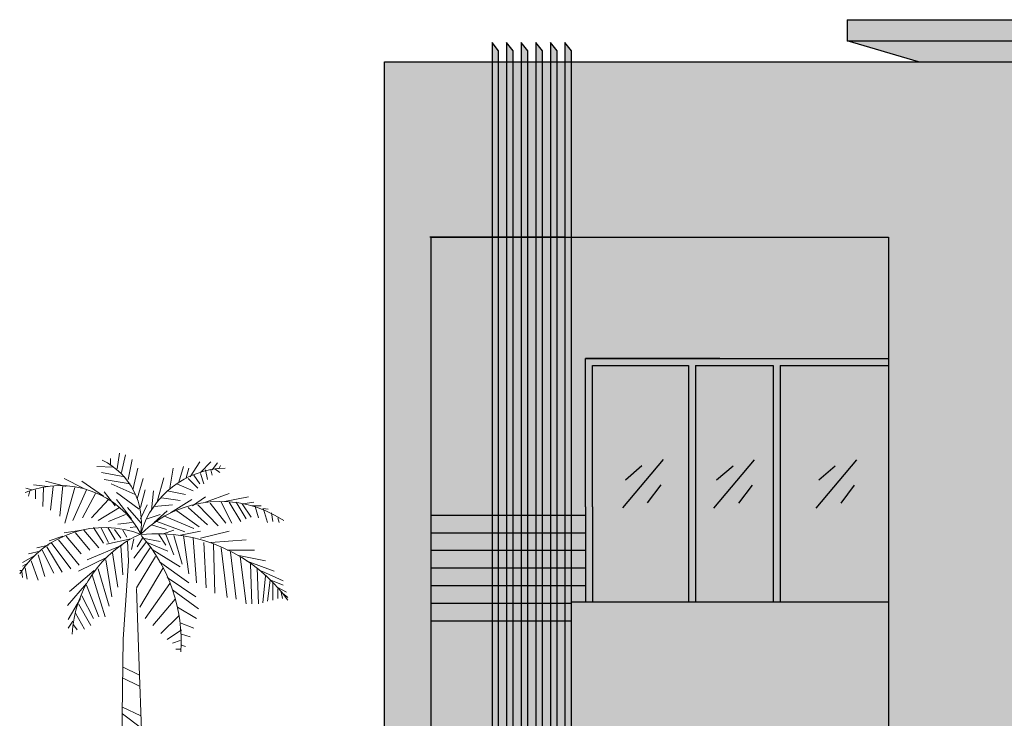
# Model space of a CAD drawing. Units: inches. Extents: x 13 to 1693, y -7 to 1519.
# Tile 6 of 10: x 13 to 292, y 1321 to 1519. Entities that reach past the tile are written whole.
import ezdxf

# ---------------------------------------------------------------- set-up
doc = ezdxf.new("R2010")
doc.units = ezdxf.units.IN
doc.header["$MEASUREMENT"] = 0
for name, color, linetype, lineweight in [('A-ELEV', 7, 'Continuous', 25), ('A-ELEV-PATT', 8, 'Continuous', 13), ('TREE', 102, 'Continuous', 18)]:
    doc.layers.add(name, color=color, linetype=linetype, lineweight=lineweight)

# ---------------------------------------------------------------- blocks, each defined once
blk = doc.blocks.new('*U29')
for p, q in [((-5.567, 196.707), (-4.987, 201.167)), ((-7.5, 199.68), (-7.5, 197.946)), ((-4.407, 195.716), (-3.247, 200.672)), ((-2.474, 193.733), (-1.315, 199.433)), ((15.116, 194.477), (17.822, 198.689)), ((18.015, 195.716), (20.914, 198.689)), ((21.301, 196.459), (22.847, 198.441)), ((-6.727, 197.202), (-11.366, 197.45)), ((-3.441, 194.477), (-10.013, 195.716)), ((-1.121, 190.759), (0.232, 196.955)), ((9.317, 191.255), (10.283, 196.955)), ((11.829, 192.99), (13.182, 197.45)), ((13.956, 194.229), (14.729, 196.955)), ((18.015, 195.468), (18.981, 192.494)), ((19.368, 196.459), (19.948, 193.733)), ((20.914, 196.459), (21.301, 194.972)), ((22.074, 196.707), (23.427, 195.716)), ((23.234, 196.707), (23.62, 197.698)), ((-20.064, 191.751), (-25.863, 193.238)), ((-15.232, 191.255), (-20.644, 193.981)), ((-9.433, 189.025), (-15.618, 193.238)), ((-1.894, 192.494), (-9.24, 193.733)), ((-0.541, 189.52), (-7.307, 192.494)), ((0.038, 188.281), (1.778, 193.981)), ((5.837, 187.786), (7.577, 194.229)), ((11.25, 192.494), (15.889, 190.512)), ((14.536, 193.981), (17.242, 191.255)), ((16.082, 194.972), (17.822, 192.494)), ((-29.729, 190.759), (-31.469, 191.255)), ((-30.309, 190.512), (-30.695, 189.025)), ((-25.283, 191.751), (-29.342, 192.246)), ((-28.763, 190.759), (-28.763, 188.281)), ((-26.443, 191.503), (-26.636, 186.051)), ((-23.737, 191.751), (-24.51, 185.06)), ((-21.031, 191.998), (-21.804, 183.325)), ((-17.551, 191.503), (-20.451, 181.343)), ((-14.265, 190.759), (-18.131, 182.086)), ((-11.753, 189.768), (-15.425, 182.83)), ((-6.147, 186.299), (-9.24, 190.264)), ((-5.76, 190.016), (0.618, 185.308)), ((1.005, 185.803), (2.358, 190.759)), ((4.098, 185.06), (4.678, 190.512)), ((8.544, 190.512), (13.763, 189.52)), ((19.368, 187.29), (26.133, 189.768)), ((-8.08, 188.034), (-12.912, 182.83)), ((-5.76, 188.034), (-1.508, 182.582)), ((6.997, 188.529), (12.216, 187.786)), ((9.51, 184.317), (15.502, 188.034)), ((15.695, 186.299), (19.368, 188.777)), ((20.721, 187.042), (25.167, 181.343)), ((23.814, 187.29), (26.907, 181.343)), ((24.78, 187.538), (31.546, 188.777)), ((26.133, 187.29), (29.419, 181.838)), ((28.066, 187.29), (30.966, 182.582)), ((29.999, 186.795), (33.092, 187.29)), ((-4.987, 185.803), (-10.979, 182.086)), ((-2.668, 185.803), (1.198, 181.343)), ((1.005, 182.582), (2.938, 186.547)), ((4.871, 186.051), (10.09, 186.547)), ((4.871, 181.591), (8.544, 184.812)), ((11.25, 184.812), (17.628, 180.352)), ((14.536, 185.803), (19.948, 180.847)), ((17.242, 186.547), (23.041, 180.599)), ((29.806, 186.795), (32.319, 183.078)), ((32.512, 186.299), (35.218, 186.299)), ((33.479, 186.051), (34.445, 182.83)), ((35.605, 185.556), (37.151, 185.308)), ((35.798, 185.308), (36.958, 181.591)), ((38.118, 184.317), (38.504, 181.838)), ((-3.247, 183.821), (-8.08, 181.838)), ((-1.315, 181.591), (-5.374, 181.095)), ((2.938, 182.582), (6.61, 183.821)), ((5.644, 181.838), (13.569, 178.865)), ((7.77, 183.325), (16.082, 179.856)), ((39.857, 182.83), (40.244, 181.591)), ((-15.618, 179.36), (-20.644, 178.617)), ((-17.358, 178.617), (-13.299, 173.661)), ((-15.038, 179.36), (-10.786, 174.404)), ((-12.332, 180.104), (-9.433, 175.643)), ((-10.206, 180.104), (-8.08, 175.891)), ((-8.273, 180.104), (-6.147, 176.635)), ((-6.34, 179.608), (-4.6, 177.13)), ((-4.021, 179.36), (-2.861, 177.378)), ((-0.348, 180.352), (-1.894, 180.104)), ((4.098, 180.847), (8.35, 179.608)), ((7.384, 178.369), (10.476, 179.36)), ((11.829, 177.874), (18.015, 179.113)), ((18.015, 177.13), (26.133, 179.113)), ((-21.031, 177.626), (-24.897, 176.387)), ((-24.317, 175.891), (-18.711, 168.457)), ((-22.191, 176.635), (-16.391, 169.448)), ((-20.064, 177.626), (-15.812, 172.67)), ((-1.701, 176.882), (-8.66, 175.396)), ((-2.668, 176.387), (-2.376, 170.594)), ((-0.928, 176.882), (-1.508, 173.909)), ((2.551, 175.891), (-0.928, 171.431)), ((1.585, 177.13), (0.038, 174.652)), ((1.585, 177.13), (6.61, 176.139)), ((2.938, 175.891), (8.737, 173.413)), ((6.224, 178.121), (8.157, 175.148)), ((8.157, 178.121), (10.476, 172.422)), ((10.476, 177.874), (12.796, 169.696)), ((13.182, 177.874), (14.729, 166.97)), ((15.889, 177.13), (16.855, 164.492)), ((18.981, 175.891), (19.561, 163.005)), ((20.914, 175.891), (30.966, 176.635)), ((-27.409, 173.413), (-30.695, 172.67)), ((-25.09, 175.148), (-28.376, 174.404)), ((-26.829, 173.661), (-23.544, 167.218)), ((-25.476, 174.652), (-21.224, 167.466)), ((-4.214, 175.148), (-14.072, 170.935)), ((-6.92, 172.917), (-5.374, 163.253)), ((-4.6, 174.9), (-4.021, 166.722)), ((3.711, 174.404), (-0.541, 167.961)), ((4.291, 173.909), (12.216, 168.953)), ((21.688, 175.396), (22.074, 161.518)), ((23.814, 174.404), (25.554, 160.279)), ((25.554, 173.661), (33.285, 173.661)), ((26.52, 173.165), (28.066, 159.784)), ((-28.956, 172.174), (-32.435, 170.192)), ((-29.922, 170.687), (-27.989, 165.235)), ((-27.989, 172.422), (-26.056, 166.227)), ((-8.466, 171.678), (-16.585, 167.713)), ((-8.853, 170.935), (-7.113, 160.527)), ((5.257, 171.926), (-0.155, 163.005)), ((6.417, 170.439), (14.729, 164.492)), ((28.839, 172.174), (36.378, 170.687)), ((29.226, 171.926), (30.966, 158.545)), ((30.966, 170.687), (38.891, 167.713)), ((-32.628, 167.961), (-33.208, 167.961)), ((-32.628, 167.713), (-32.435, 165.979)), ((-31.082, 169.944), (-32.435, 169.2)), ((-31.662, 168.705), (-31.082, 165.483)), ((-12.139, 167.961), (-19.098, 162.014)), ((-10.979, 168.457), (-7.887, 157.801)), ((7.384, 168.705), (0.812, 157.553)), ((32.126, 169.696), (32.512, 158.545)), ((34.058, 168.705), (34.445, 158.545)), ((35.412, 167.713), (41.404, 164.988)), ((-12.719, 166.722), (-9.046, 154.828)), ((8.544, 165.979), (16.662, 160.527)), ((36.378, 166.474), (35.605, 158.792)), ((37.731, 165.235), (36.958, 159.288)), ((37.924, 165.235), (41.404, 163.749)), ((-14.265, 164.244), (-19.678, 158.049)), ((-14.265, 163.749), (-10.786, 154.828)), ((9.317, 164.244), (2.358, 154.332)), ((10.09, 162.51), (17.435, 157.058)), ((38.504, 164.492), (38.504, 159.536)), ((39.664, 163.253), (42.37, 161.766)), ((39.857, 162.757), (39.857, 160.031)), ((40.824, 161.766), (41.21, 160.031)), ((-16.005, 160.031), (-19.484, 154.084)), ((-15.618, 160.775), (-12.332, 154.332)), ((10.863, 159.784), (4.484, 152.35)), ((41.21, 161.518), (42.757, 160.279)), ((-16.585, 158.545), (-13.106, 152.35)), ((11.443, 157.553), (16.855, 154.332)), ((-18.131, 153.589), (-19.484, 151.606)), ((-17.358, 155.819), (-14.845, 151.358)), ((11.829, 155.075), (6.804, 150.119)), ((-17.938, 152.597), (-16.972, 151.111)), ((12.603, 151.111), (8.544, 148.385)), ((12.216, 153.093), (16.082, 151.606)), ((12.216, 148.137), (10.09, 147.393)), ((12.603, 149.872), (15.116, 149.128)), ((12.409, 145.659), (11.056, 145.659)), ((12.409, 146.898), (13.763, 146.402)), ((-4.081, 140.645), (0.753, 138.261)), ((-4.081, 137.547), (0.753, 135.163)), ((-4.081, 129.205), (1.124, 126.821)), ((-4.081, 127.298), (1.31, 123.246)), ((-4.081, 121.578), (1.31, 120.863)), ((-4.267, 114.428), (1.682, 108.708)), ((-4.453, 112.283), (1.682, 105.133)), ((-4.639, 102.273), (1.868, 100.604)), ((-4.453, 99.651), (2.24, 98.459)), ((-4.453, 91.071), (2.426, 89.641)), ((-4.825, 83.921), (2.612, 81.061)), ((-4.639, 81.299), (2.797, 78.916)), ((-4.639, 78.916), (2.797, 76.771))]:
    blk.add_line(p, q)
for points in [[(-2.363, 170.553), (-3.88, 148.505), (-4.988, 69.634), (-3.325, 24.869), (0, 0)], [(-0.116, 162.848), (0.554, 143.532), (2.217, 96.635), (3.88, 44.054), (7.76, 12.079), (11.64, 0)]]:
    blk.add_lwpolyline(points)
for centre, radius, start, end in [((-18.427, 181.448), 19.715, 350.285, 64.11229), ((25.595, 171.567), 25.395, 91.40319, 163.882), ((-21.738, 166.094), 25.899, 27.67115, 112.5305), ((23.687, 155.341), 32.188, 56.19272, 134.3213), ((-9.259, 151.732), 28.386, 68.38311, 147.5322), ((14.394, 148.393), 32.752, 113.7592, 177.4133), ((5.828, 132.718), 45.639, 35.98777, 95.82273), ((-32.8, 147.923), 45.309, 356.1943, 41.37848)]:
    blk.add_arc(centre, radius, start, end)

msp = doc.modelspace()

# ---------------------------------------------------------------- hatches: boundary and pattern name
at = {"layer": 'A-ELEV-PATT'}
h = msp.add_hatch(color=256, dxfattribs=at)
h.dxf.hatch_style = 1
h.paths.add_polyline_path([(526.9, 1519.22), (247.4, 1519.22), (247.4, 1513.22), (526.9, 1513.22)])
at = {"layer": 'A-ELEV-PATT', "transparency": 33554664}
h = msp.add_hatch(color=256, dxfattribs=at)
h.dxf.hatch_style = 1
h.paths.add_polyline_path([(161.14, 1507.23), (159.26, 1507.23), (159.26, 1457.61), (161.14, 1457.61)])
h.paths.add_polyline_path([(161.14, 1510.4), (159.26, 1512.79), (159.26, 1507.23), (161.14, 1507.23)])
h.paths.add_polyline_path([(165.27, 1510.4), (163.39, 1512.79), (163.39, 1507.23), (165.27, 1507.23)])
h.paths.add_polyline_path([(169.4, 1510.4), (167.53, 1512.79), (167.53, 1507.23), (169.4, 1507.23)])
h.paths.add_polyline_path([(157.01, 1510.4), (155.13, 1512.79), (155.13, 1507.23), (157.01, 1507.23)])
h.paths.add_polyline_path([(152.87, 1510.4), (151, 1512.79), (151, 1507.23), (152.87, 1507.23)])
h.paths.add_polyline_path([(148.74, 1510.4), (146.87, 1512.79), (146.87, 1507.23), (148.74, 1507.23)])
h.paths.add_polyline_path([(148.74, 1507.23), (146.87, 1507.23), (146.87, 1457.61), (148.74, 1457.61)])
h.paths.add_polyline_path([(152.87, 1507.23), (151, 1507.23), (151, 1457.61), (152.87, 1457.61)])
h.paths.add_polyline_path([(157.01, 1507.23), (155.13, 1507.23), (155.13, 1457.61), (157.01, 1457.61)])
h.paths.add_polyline_path([(165.27, 1507.23), (163.39, 1507.23), (163.39, 1457.61), (165.27, 1457.61)])
h.paths.add_polyline_path([(169.4, 1507.23), (167.53, 1507.23), (167.53, 1457.61), (169.4, 1457.61)])
h.paths.add_polyline_path([(157.01, 1457.61), (155.13, 1457.61), (155.13, 1213.23), (157.01, 1213.23)])
h.paths.add_polyline_path([(161.14, 1457.61), (159.26, 1457.61), (159.26, 1213.23), (161.14, 1213.23)])
h.paths.add_polyline_path([(165.27, 1457.61), (163.39, 1457.61), (163.39, 1213.23), (165.27, 1213.23)])
h.paths.add_polyline_path([(169.4, 1457.61), (167.53, 1457.61), (167.53, 1213.23), (169.4, 1213.23)])
h.paths.add_polyline_path([(152.87, 1457.61), (151, 1457.61), (151, 1213.23), (152.87, 1213.23)])
h.paths.add_polyline_path([(148.74, 1457.61), (146.87, 1457.61), (146.87, 1213.23), (148.74, 1213.23)])
at = {"layer": 'A-ELEV-PATT'}
h = msp.add_hatch(color=256, dxfattribs=at)
h.dxf.hatch_style = 1
h.paths.add_polyline_path([(485.45, 1459.23), (314.45, 1459.23), (323.77, 1437.38), (485.45, 1437.38)])
h.paths.add_polyline_path([(323.77, 1437.38), (314.45, 1459.23), (314.45, 1204.63), (323.77, 1213.23), (323.77, 1423.23)])
h.paths.add_polyline_path([(526.9, 1513.22), (247.4, 1513.22), (267.64, 1507.23), (519.7, 1507.23)])
h = msp.add_hatch(color=256, dxfattribs=at)
h.dxf.hatch_style = 1
h.paths.add_polyline_path([(534.67, 1493.81), (311.73, 1493.81), (311.73, 1507.23), (169.4, 1507.23), (169.4, 1457.61), (259.19, 1457.61), (259.19, 1213.23), (294.63, 1213.23), (294.63, 1485.7), (299.21, 1485.7), (534.67, 1485.7)])
h.paths.add_polyline_path([(534.67, 1481.12), (299.21, 1481.12), (299.21, 1213.23), (314.45, 1213.23), (314.45, 1459.23), (520.13, 1459.23)], flags=17)
h.paths.add_polyline_path([(146.87, 1507.23), (116.45, 1507.23), (116.45, 1339.23), (116.45, 1213.23), (129.66, 1213.23), (129.66, 1457.61), (146.87, 1457.61)])
h.paths.add_polyline_path([(151, 1507.23), (148.74, 1507.23), (148.74, 1457.61), (151, 1457.61)])
h.paths.add_polyline_path([(155.13, 1507.23), (152.87, 1507.23), (152.87, 1457.61), (155.13, 1457.61)])
h.paths.add_polyline_path([(159.26, 1507.23), (157.01, 1507.23), (157.01, 1457.61), (159.26, 1457.61)])
h.paths.add_polyline_path([(163.39, 1507.23), (161.14, 1507.23), (161.14, 1457.61), (163.39, 1457.61)])
h.paths.add_polyline_path([(167.53, 1507.23), (165.27, 1507.23), (165.27, 1457.61), (167.53, 1457.61)])
h = msp.add_hatch(color=256, dxfattribs=at)
h.dxf.hatch_style = 1
h.paths.add_polyline_path([(259.19, 1457.61), (169.4, 1457.61), (169.4, 1453.8), (259.19, 1453.8)])
h.paths.add_polyline_path([(259.19, 1448.8), (169.4, 1448.8), (169.4, 1443.8), (259.19, 1443.8)])
h.paths.add_polyline_path([(259.19, 1438.8), (169.4, 1438.8), (169.4, 1433.8), (259.19, 1433.8)])
h.paths.add_polyline_path([(259.19, 1428.8), (169.4, 1428.8), (169.4, 1423.8), (259.19, 1423.8)])
h.paths.add_polyline_path([(146.87, 1457.61), (129.66, 1457.61), (129.66, 1453.8), (146.87, 1453.8)])
h.paths.add_polyline_path([(146.87, 1448.8), (129.66, 1448.8), (129.66, 1443.8), (146.87, 1443.8)])
h.paths.add_polyline_path([(146.87, 1438.8), (129.66, 1438.8), (129.66, 1433.8), (146.87, 1433.8)])
h.paths.add_polyline_path([(146.87, 1428.8), (129.66, 1428.8), (129.66, 1423.8), (146.87, 1423.8)])
h.paths.add_polyline_path([(151, 1457.61), (148.74, 1457.61), (148.74, 1453.8), (151, 1453.8)])
h.paths.add_polyline_path([(155.13, 1457.61), (152.87, 1457.61), (152.87, 1453.8), (155.13, 1453.8)])
h.paths.add_polyline_path([(159.26, 1457.61), (157.01, 1457.61), (157.01, 1453.8), (159.26, 1453.8)])
h.paths.add_polyline_path([(163.39, 1457.61), (161.14, 1457.61), (161.14, 1453.8), (163.39, 1453.8)])
h.paths.add_polyline_path([(167.53, 1457.61), (165.27, 1457.61), (165.27, 1453.8), (167.53, 1453.8)])
h.paths.add_polyline_path([(167.53, 1448.8), (165.27, 1448.8), (165.27, 1443.8), (167.53, 1443.8)])
h.paths.add_polyline_path([(163.39, 1448.8), (161.14, 1448.8), (161.14, 1443.8), (163.39, 1443.8)])
h.paths.add_polyline_path([(159.26, 1448.8), (157.01, 1448.8), (157.01, 1443.8), (159.26, 1443.8)])
h.paths.add_polyline_path([(155.13, 1448.8), (152.87, 1448.8), (152.87, 1443.8), (155.13, 1443.8)])
h.paths.add_polyline_path([(151, 1448.8), (148.74, 1448.8), (148.74, 1443.8), (151, 1443.8)])
h.paths.add_polyline_path([(151, 1438.8), (148.74, 1438.8), (148.74, 1433.8), (151, 1433.8)])
h.paths.add_polyline_path([(155.13, 1438.8), (152.87, 1438.8), (152.87, 1433.8), (155.13, 1433.8)])
h.paths.add_polyline_path([(159.26, 1438.8), (157.01, 1438.8), (157.01, 1433.8), (159.26, 1433.8)])
h.paths.add_polyline_path([(163.39, 1438.8), (161.14, 1438.8), (161.14, 1433.8), (163.39, 1433.8)])
h.paths.add_polyline_path([(167.53, 1438.8), (165.27, 1438.8), (165.27, 1433.8), (167.53, 1433.8)])
h.paths.add_polyline_path([(167.53, 1428.8), (165.27, 1428.8), (165.27, 1423.8), (167.53, 1423.8)])
h.paths.add_polyline_path([(163.39, 1428.8), (161.14, 1428.8), (161.14, 1423.8), (163.39, 1423.8)])
h.paths.add_polyline_path([(159.26, 1428.8), (157.01, 1428.8), (157.01, 1423.8), (159.26, 1423.8)])
h.paths.add_polyline_path([(155.13, 1428.8), (152.87, 1428.8), (152.87, 1423.8), (155.13, 1423.8)])
h.paths.add_polyline_path([(151, 1428.8), (148.74, 1428.8), (148.74, 1423.8), (151, 1423.8)])
h.paths.add_polyline_path([(146.87, 1418.8), (129.66, 1418.8), (129.66, 1413.8), (146.87, 1413.8)])
h.paths.add_polyline_path([(146.87, 1408.8), (129.66, 1408.8), (129.66, 1403.8), (146.87, 1403.8)])
h.paths.add_polyline_path([(146.87, 1398.8), (129.66, 1398.8), (129.66, 1393.8), (146.87, 1393.8)])
h.paths.add_polyline_path([(146.87, 1388.8), (129.66, 1388.8), (129.66, 1383.8), (146.87, 1383.8)])
h.paths.add_polyline_path([(146.87, 1378.8), (129.66, 1378.8), (129.66, 1373.8), (146.87, 1373.8)])
h.paths.add_polyline_path([(146.87, 1368.8), (129.66, 1368.8), (129.66, 1363.8), (146.87, 1363.8)])
h.paths.add_polyline_path([(146.87, 1358.8), (129.66, 1358.8), (129.66, 1353.8), (146.87, 1353.8)])
h.paths.add_polyline_path([(146.87, 1348.8), (129.66, 1348.8), (129.66, 1343.8), (146.87, 1343.8)])
h.paths.add_polyline_path([(146.87, 1338.8), (129.66, 1338.8), (129.66, 1333.8), (146.87, 1333.8)])
h.paths.add_polyline_path([(146.87, 1328.8), (129.66, 1328.8), (129.66, 1323.8), (146.87, 1323.8)])
h.paths.add_polyline_path([(146.87, 1318.8), (129.66, 1318.8), (129.66, 1312.21), (146.87, 1312.21)])
h.paths.add_polyline_path([(146.87, 1307.21), (129.66, 1307.21), (129.66, 1302.21), (146.87, 1302.21)])
h.paths.add_polyline_path([(146.87, 1297.21), (129.66, 1297.21), (129.66, 1292.21), (146.87, 1292.21)])
h.paths.add_polyline_path([(146.87, 1287.21), (129.66, 1287.21), (129.66, 1282.21), (146.87, 1282.21)])
h.paths.add_polyline_path([(146.87, 1277.21), (129.66, 1277.21), (129.66, 1272.21), (146.87, 1272.21)])
h.paths.add_polyline_path([(146.87, 1267.21), (129.66, 1267.21), (129.66, 1262.21), (146.87, 1262.21)])
h.paths.add_polyline_path([(146.87, 1257.21), (129.66, 1257.21), (129.66, 1252.21), (146.87, 1252.21)])
h.paths.add_polyline_path([(146.87, 1247.21), (129.66, 1247.21), (129.66, 1242.21), (146.87, 1242.21)])
h = msp.add_hatch(color=256, dxfattribs=at)
h.dxf.hatch_style = 1
h.paths.add_polyline_path([(259.19, 1453.8), (169.4, 1453.8), (169.4, 1448.8), (259.19, 1448.8)])
h.paths.add_polyline_path([(259.19, 1443.8), (169.4, 1443.8), (169.4, 1438.8), (259.19, 1438.8)])
h.paths.add_polyline_path([(259.19, 1433.8), (169.4, 1433.8), (169.4, 1428.8), (259.19, 1428.8)])
h.paths.add_polyline_path([(146.87, 1453.8), (129.66, 1453.8), (129.66, 1448.8), (146.87, 1448.8)])
h.paths.add_polyline_path([(146.87, 1443.8), (129.66, 1443.8), (129.66, 1438.8), (146.87, 1438.8)])
h.paths.add_polyline_path([(146.87, 1433.8), (129.66, 1433.8), (129.66, 1428.8), (146.87, 1428.8)])
h.paths.add_polyline_path([(146.87, 1423.8), (129.66, 1423.8), (129.66, 1418.8), (146.87, 1418.8)])
h.paths.add_polyline_path([(146.87, 1413.8), (129.66, 1413.8), (129.66, 1408.8), (146.87, 1408.8)])
h.paths.add_polyline_path([(146.87, 1403.8), (129.66, 1403.8), (129.66, 1398.8), (146.87, 1398.8)])
h.paths.add_polyline_path([(146.87, 1393.8), (129.66, 1393.8), (129.66, 1388.8), (146.87, 1388.8)])
h.paths.add_polyline_path([(146.87, 1383.8), (129.66, 1383.8), (129.66, 1378.8), (146.87, 1378.8)])
h.paths.add_polyline_path([(146.87, 1373.8), (129.66, 1373.8), (129.66, 1368.8), (146.87, 1368.8)])
h.paths.add_polyline_path([(146.87, 1363.8), (129.66, 1363.8), (129.66, 1358.8), (146.87, 1358.8)])
h.paths.add_polyline_path([(146.87, 1353.8), (129.66, 1353.8), (129.66, 1348.8), (146.87, 1348.8)])
h.paths.add_polyline_path([(146.87, 1343.8), (129.66, 1343.8), (129.66, 1338.8), (146.87, 1338.8)])
h.paths.add_polyline_path([(146.87, 1333.8), (129.66, 1333.8), (129.66, 1328.8), (146.87, 1328.8)])
h.paths.add_polyline_path([(146.87, 1323.8), (129.66, 1323.8), (129.66, 1318.8), (146.87, 1318.8)])
h.paths.add_polyline_path([(146.87, 1312.21), (129.66, 1312.21), (129.66, 1307.21), (146.87, 1307.21)])
h.paths.add_polyline_path([(146.87, 1302.21), (129.66, 1302.21), (129.66, 1297.21), (146.87, 1297.21)])
h.paths.add_polyline_path([(146.87, 1292.21), (129.66, 1292.21), (129.66, 1287.21), (146.87, 1287.21)])
h.paths.add_polyline_path([(146.87, 1282.21), (129.66, 1282.21), (129.66, 1277.21), (146.87, 1277.21)])
h.paths.add_polyline_path([(146.87, 1272.21), (129.66, 1272.21), (129.66, 1267.21), (146.87, 1267.21)])
h.paths.add_polyline_path([(146.87, 1262.21), (129.66, 1262.21), (129.66, 1257.21), (146.87, 1257.21)])
h.paths.add_polyline_path([(146.87, 1252.21), (129.66, 1252.21), (129.66, 1247.21), (146.87, 1247.21)])
h.paths.add_polyline_path([(146.87, 1242.21), (129.66, 1242.21), (129.66, 1237.21), (146.87, 1237.21)])
h.paths.add_polyline_path([(146.87, 1232.21), (129.66, 1232.21), (129.66, 1227.21), (146.87, 1227.21)])
h.paths.add_polyline_path([(146.87, 1222.21), (129.66, 1222.21), (129.66, 1217.21), (146.87, 1217.21)])
h.paths.add_polyline_path([(259.19, 1242.21), (169.4, 1242.21), (169.4, 1237.21), (259.19, 1237.21)])
h.paths.add_polyline_path([(259.19, 1232.21), (169.4, 1232.21), (169.4, 1227.21), (259.19, 1227.21)])
h.paths.add_polyline_path([(259.19, 1222.21), (169.4, 1222.21), (169.4, 1217.21), (259.19, 1217.21)])
h = msp.add_hatch(color=256, dxfattribs=at)
h.dxf.hatch_style = 1
h.paths.add_polyline_path([(173.34, 1282.21), (169.4, 1282.21), (169.4, 1277.21), (173.34, 1277.21)])
h.paths.add_polyline_path([(173.34, 1292.21), (169.4, 1292.21), (169.4, 1287.21), (173.34, 1287.21)])
h.paths.add_polyline_path([(173.34, 1272.21), (169.4, 1272.21), (169.4, 1267.21), (173.34, 1267.21)])
h.paths.add_polyline_path([(173.34, 1262.21), (169.4, 1262.21), (169.4, 1257.21), (173.34, 1257.21)])
h.paths.add_polyline_path([(173.34, 1312.21), (169.4, 1312.21), (169.4, 1307.21), (173.34, 1307.21)])
h.paths.add_polyline_path([(173.34, 1302.21), (169.4, 1302.21), (169.4, 1297.21), (173.34, 1297.21)])
h.paths.add_polyline_path([(167.53, 1323.8), (165.27, 1323.8), (165.27, 1318.8), (167.53, 1318.8)])
h.paths.add_polyline_path([(167.53, 1333.8), (165.27, 1333.8), (165.27, 1328.8), (167.53, 1328.8)])
h.paths.add_polyline_path([(163.39, 1333.8), (161.14, 1333.8), (161.14, 1328.8), (163.39, 1328.8)])
h.paths.add_polyline_path([(159.26, 1333.8), (157.01, 1333.8), (157.01, 1328.8), (159.26, 1328.8)])
h.paths.add_polyline_path([(155.13, 1333.8), (152.87, 1333.8), (152.87, 1328.8), (155.13, 1328.8)])
h.paths.add_polyline_path([(151, 1333.8), (148.74, 1333.8), (148.74, 1328.8), (151, 1328.8)])
h.paths.add_polyline_path([(151, 1323.8), (148.74, 1323.8), (148.74, 1318.8), (151, 1318.8)])
h.paths.add_polyline_path([(155.13, 1323.8), (152.87, 1323.8), (152.87, 1318.8), (155.13, 1318.8)])
h.paths.add_polyline_path([(159.26, 1323.8), (157.01, 1323.8), (157.01, 1318.8), (159.26, 1318.8)])
h.paths.add_polyline_path([(163.39, 1323.8), (161.14, 1323.8), (161.14, 1318.8), (163.39, 1318.8)])
h.paths.add_polyline_path([(163.39, 1312.21), (161.14, 1312.21), (161.14, 1307.21), (163.39, 1307.21)])
h.paths.add_polyline_path([(167.53, 1312.21), (165.27, 1312.21), (165.27, 1307.21), (167.53, 1307.21)])
h.paths.add_polyline_path([(167.53, 1302.21), (165.27, 1302.21), (165.27, 1297.21), (167.53, 1297.21)])
h.paths.add_polyline_path([(167.53, 1292.21), (165.27, 1292.21), (165.27, 1287.21), (167.53, 1287.21)])
h.paths.add_polyline_path([(163.39, 1292.21), (161.14, 1292.21), (161.14, 1287.21), (163.39, 1287.21)])
h.paths.add_polyline_path([(163.39, 1302.21), (161.14, 1302.21), (161.14, 1297.21), (163.39, 1297.21)])
h.paths.add_polyline_path([(159.26, 1302.21), (157.01, 1302.21), (157.01, 1297.21), (159.26, 1297.21)])
h.paths.add_polyline_path([(159.26, 1312.21), (157.01, 1312.21), (157.01, 1307.21), (159.26, 1307.21)])
h.paths.add_polyline_path([(155.13, 1312.21), (152.87, 1312.21), (152.87, 1307.21), (155.13, 1307.21)])
h.paths.add_polyline_path([(151, 1312.21), (148.74, 1312.21), (148.74, 1307.21), (151, 1307.21)])
h.paths.add_polyline_path([(151, 1302.21), (148.74, 1302.21), (148.74, 1297.21), (151, 1297.21)])
h.paths.add_polyline_path([(155.13, 1302.21), (152.87, 1302.21), (152.87, 1297.21), (155.13, 1297.21)])
h.paths.add_polyline_path([(155.13, 1292.21), (152.87, 1292.21), (152.87, 1287.21), (155.13, 1287.21)])
h.paths.add_polyline_path([(151, 1292.21), (148.74, 1292.21), (148.74, 1287.21), (151, 1287.21)])
h.paths.add_polyline_path([(159.26, 1292.21), (157.01, 1292.21), (157.01, 1287.21), (159.26, 1287.21)])
h.paths.add_polyline_path([(159.26, 1282.21), (157.01, 1282.21), (157.01, 1277.21), (159.26, 1277.21)])
h.paths.add_polyline_path([(163.39, 1282.21), (161.14, 1282.21), (161.14, 1277.21), (163.39, 1277.21)])
h.paths.add_polyline_path([(167.53, 1282.21), (165.27, 1282.21), (165.27, 1277.21), (167.53, 1277.21)])
h.paths.add_polyline_path([(155.13, 1282.21), (152.87, 1282.21), (152.87, 1277.21), (155.13, 1277.21)])
h.paths.add_polyline_path([(151, 1282.21), (148.74, 1282.21), (148.74, 1277.21), (151, 1277.21)])
h.paths.add_polyline_path([(151, 1272.21), (148.74, 1272.21), (148.74, 1267.21), (151, 1267.21)])
h.paths.add_polyline_path([(155.13, 1272.21), (152.87, 1272.21), (152.87, 1267.21), (155.13, 1267.21)])
h.paths.add_polyline_path([(159.26, 1272.21), (157.01, 1272.21), (157.01, 1267.21), (159.26, 1267.21)])
h.paths.add_polyline_path([(163.39, 1272.21), (161.14, 1272.21), (161.14, 1267.21), (163.39, 1267.21)])
h.paths.add_polyline_path([(167.53, 1272.21), (165.27, 1272.21), (165.27, 1267.21), (167.53, 1267.21)])
h.paths.add_polyline_path([(167.53, 1262.21), (165.27, 1262.21), (165.27, 1257.21), (167.53, 1257.21)])
h.paths.add_polyline_path([(163.39, 1262.21), (161.14, 1262.21), (161.14, 1257.21), (163.39, 1257.21)])
h.paths.add_polyline_path([(163.39, 1252.21), (161.14, 1252.21), (161.14, 1247.21), (163.39, 1247.21)])
h.paths.add_polyline_path([(159.26, 1252.21), (157.01, 1252.21), (157.01, 1247.21), (159.26, 1247.21)])
h.paths.add_polyline_path([(159.26, 1262.21), (157.01, 1262.21), (157.01, 1257.21), (159.26, 1257.21)])
h.paths.add_polyline_path([(155.13, 1262.21), (152.87, 1262.21), (152.87, 1257.21), (155.13, 1257.21)])
h.paths.add_polyline_path([(151, 1262.21), (148.74, 1262.21), (148.74, 1257.21), (151, 1257.21)])
h.paths.add_polyline_path([(151, 1252.21), (148.74, 1252.21), (148.74, 1247.21), (151, 1247.21)])
h.paths.add_polyline_path([(155.13, 1252.21), (152.87, 1252.21), (152.87, 1247.21), (155.13, 1247.21)])
h.paths.add_polyline_path([(151, 1242.21), (148.74, 1242.21), (148.74, 1237.21), (151, 1237.21)])
h.paths.add_polyline_path([(155.13, 1242.21), (152.87, 1242.21), (152.87, 1237.21), (155.13, 1237.21)])
h.paths.add_polyline_path([(159.26, 1242.21), (157.01, 1242.21), (157.01, 1237.21), (159.26, 1237.21)])
h.paths.add_polyline_path([(163.39, 1242.21), (161.14, 1242.21), (161.14, 1237.21), (163.39, 1237.21)])
h.paths.add_polyline_path([(173.34, 1363.8), (169.4, 1363.8), (169.4, 1358.8), (173.34, 1358.8)])
h.paths.add_polyline_path([(173.34, 1373.8), (169.4, 1373.8), (169.4, 1368.8), (173.34, 1368.8)])
h.paths.add_polyline_path([(173.34, 1381.23), (173.34, 1383.8), (169.4, 1383.8), (169.4, 1378.8), (173.34, 1378.8)])
h.paths.add_polyline_path([(173.34, 1393.8), (169.4, 1393.8), (169.4, 1388.8), (173.34, 1388.8)])
h.paths.add_polyline_path([(173.34, 1403.8), (169.4, 1403.8), (169.4, 1398.8), (173.34, 1398.8)])
h.paths.add_polyline_path([(173.34, 1413.8), (169.4, 1413.8), (169.4, 1408.8), (173.34, 1408.8)])
h.paths.add_polyline_path([(167.53, 1383.8), (165.27, 1383.8), (165.27, 1378.8), (167.53, 1378.8)])
h.paths.add_polyline_path([(167.53, 1373.8), (165.27, 1373.8), (165.27, 1368.8), (167.53, 1368.8)])
h.paths.add_polyline_path([(167.53, 1363.8), (165.27, 1363.8), (165.27, 1358.8), (167.53, 1358.8)])
h.paths.add_polyline_path([(167.53, 1353.8), (165.27, 1353.8), (165.27, 1348.8), (167.53, 1348.8)])
h.paths.add_polyline_path([(163.39, 1353.8), (161.14, 1353.8), (161.14, 1348.8), (163.39, 1348.8)])
h.paths.add_polyline_path([(163.39, 1363.8), (161.14, 1363.8), (161.14, 1358.8), (163.39, 1358.8)])
h.paths.add_polyline_path([(163.39, 1373.8), (161.14, 1373.8), (161.14, 1368.8), (163.39, 1368.8)])
h.paths.add_polyline_path([(163.39, 1383.8), (161.14, 1383.8), (161.14, 1378.8), (163.39, 1378.8)])
h.paths.add_polyline_path([(163.39, 1393.8), (161.14, 1393.8), (161.14, 1388.8), (163.39, 1388.8)])
h.paths.add_polyline_path([(163.39, 1403.8), (161.14, 1403.8), (161.14, 1398.8), (163.39, 1398.8)])
h.paths.add_polyline_path([(167.53, 1403.8), (165.27, 1403.8), (165.27, 1398.8), (167.53, 1398.8)])
h.paths.add_polyline_path([(167.53, 1393.8), (165.27, 1393.8), (165.27, 1388.8), (167.53, 1388.8)])
h.paths.add_polyline_path([(167.53, 1413.8), (165.27, 1413.8), (165.27, 1408.8), (167.53, 1408.8)])
h.paths.add_polyline_path([(163.39, 1413.8), (161.14, 1413.8), (161.14, 1408.8), (163.39, 1408.8)])
h.paths.add_polyline_path([(159.26, 1413.8), (157.01, 1413.8), (157.01, 1408.8), (159.26, 1408.8)])
h.paths.add_polyline_path([(155.13, 1413.8), (152.87, 1413.8), (152.87, 1408.8), (155.13, 1408.8)])
h.paths.add_polyline_path([(151, 1413.8), (148.74, 1413.8), (148.74, 1408.8), (151, 1408.8)])
h.paths.add_polyline_path([(151, 1403.8), (148.74, 1403.8), (148.74, 1398.8), (151, 1398.8)])
h.paths.add_polyline_path([(155.13, 1403.8), (152.87, 1403.8), (152.87, 1398.8), (155.13, 1398.8)])
h.paths.add_polyline_path([(159.26, 1403.8), (157.01, 1403.8), (157.01, 1398.8), (159.26, 1398.8)])
h.paths.add_polyline_path([(159.26, 1393.8), (157.01, 1393.8), (157.01, 1388.8), (159.26, 1388.8)])
h.paths.add_polyline_path([(155.13, 1393.8), (152.87, 1393.8), (152.87, 1388.8), (155.13, 1388.8)])
h.paths.add_polyline_path([(151, 1393.8), (148.74, 1393.8), (148.74, 1388.8), (151, 1388.8)])
h.paths.add_polyline_path([(151, 1383.8), (148.74, 1383.8), (148.74, 1378.8), (151, 1378.8)])
h.paths.add_polyline_path([(155.13, 1383.8), (152.87, 1383.8), (152.87, 1378.8), (155.13, 1378.8)])
h.paths.add_polyline_path([(159.26, 1383.8), (157.01, 1383.8), (157.01, 1378.8), (159.26, 1378.8)])
h.paths.add_polyline_path([(159.26, 1373.8), (157.01, 1373.8), (157.01, 1368.8), (159.26, 1368.8)])
h.paths.add_polyline_path([(155.13, 1373.8), (152.87, 1373.8), (152.87, 1368.8), (155.13, 1368.8)])
h.paths.add_polyline_path([(151, 1373.8), (148.74, 1373.8), (148.74, 1368.8), (151, 1368.8)])
h.paths.add_polyline_path([(151, 1363.8), (148.74, 1363.8), (148.74, 1358.8), (151, 1358.8)])
h.paths.add_polyline_path([(155.13, 1363.8), (152.87, 1363.8), (152.87, 1358.8), (155.13, 1358.8)])
h.paths.add_polyline_path([(159.26, 1363.8), (157.01, 1363.8), (157.01, 1358.8), (159.26, 1358.8)])
h.paths.add_polyline_path([(159.26, 1353.8), (157.01, 1353.8), (157.01, 1348.8), (159.26, 1348.8)])
h.paths.add_polyline_path([(155.13, 1353.8), (152.87, 1353.8), (152.87, 1348.8), (155.13, 1348.8)])
h.paths.add_polyline_path([(151, 1353.8), (148.74, 1353.8), (148.74, 1348.8), (151, 1348.8)])
h.paths.add_polyline_path([(151, 1343.8), (148.74, 1343.8), (148.74, 1338.8), (151, 1338.8)])
h.paths.add_polyline_path([(155.13, 1343.8), (152.87, 1343.8), (152.87, 1338.8), (155.13, 1338.8)])
h.paths.add_polyline_path([(159.26, 1343.8), (157.01, 1343.8), (157.01, 1338.8), (159.26, 1338.8)])
h.paths.add_polyline_path([(163.39, 1343.8), (161.14, 1343.8), (161.14, 1338.8), (163.39, 1338.8)])
h.paths.add_polyline_path([(167.53, 1343.8), (165.27, 1343.8), (165.27, 1338.8), (167.53, 1338.8)])
h.paths.add_polyline_path([(151, 1453.8), (148.74, 1453.8), (148.74, 1448.8), (151, 1448.8)])
h.paths.add_polyline_path([(155.13, 1453.8), (152.87, 1453.8), (152.87, 1448.8), (155.13, 1448.8)])
h.paths.add_polyline_path([(159.26, 1453.8), (157.01, 1453.8), (157.01, 1448.8), (159.26, 1448.8)])
h.paths.add_polyline_path([(163.39, 1453.8), (161.14, 1453.8), (161.14, 1448.8), (163.39, 1448.8)])
h.paths.add_polyline_path([(167.53, 1453.8), (165.27, 1453.8), (165.27, 1448.8), (167.53, 1448.8)])
h.paths.add_polyline_path([(167.53, 1443.8), (165.27, 1443.8), (165.27, 1438.8), (167.53, 1438.8)])
h.paths.add_polyline_path([(163.39, 1443.8), (161.14, 1443.8), (161.14, 1438.8), (163.39, 1438.8)])
h.paths.add_polyline_path([(159.26, 1443.8), (157.01, 1443.8), (157.01, 1438.8), (159.26, 1438.8)])
h.paths.add_polyline_path([(155.13, 1443.8), (152.87, 1443.8), (152.87, 1438.8), (155.13, 1438.8)])
h.paths.add_polyline_path([(151, 1443.8), (148.74, 1443.8), (148.74, 1438.8), (151, 1438.8)])
h.paths.add_polyline_path([(151, 1433.8), (148.74, 1433.8), (148.74, 1428.8), (151, 1428.8)])
h.paths.add_polyline_path([(155.13, 1433.8), (152.87, 1433.8), (152.87, 1428.8), (155.13, 1428.8)])
h.paths.add_polyline_path([(159.26, 1433.8), (157.01, 1433.8), (157.01, 1428.8), (159.26, 1428.8)])
h.paths.add_polyline_path([(163.39, 1433.8), (161.14, 1433.8), (161.14, 1428.8), (163.39, 1428.8)])
h.paths.add_polyline_path([(167.53, 1433.8), (165.27, 1433.8), (165.27, 1428.8), (167.53, 1428.8)])
h.paths.add_polyline_path([(173.34, 1423.23), (249.37, 1423.23), (259.19, 1423.23), (259.19, 1423.8), (169.4, 1423.8), (169.4, 1418.8), (173.34, 1418.8)])
h.paths.add_polyline_path([(167.53, 1423.8), (165.27, 1423.8), (165.27, 1418.8), (167.53, 1418.8)])
h.paths.add_polyline_path([(163.39, 1423.8), (161.14, 1423.8), (161.14, 1418.8), (163.39, 1418.8)])
h.paths.add_polyline_path([(159.26, 1423.8), (157.01, 1423.8), (157.01, 1418.8), (159.26, 1418.8)])
h.paths.add_polyline_path([(155.13, 1423.8), (152.87, 1423.8), (152.87, 1418.8), (155.13, 1418.8)])
h.paths.add_polyline_path([(151, 1423.8), (148.74, 1423.8), (148.74, 1418.8), (151, 1418.8)])
h = msp.add_hatch(color=256, dxfattribs=at)
h.dxf.hatch_style = 1
h.paths.add_polyline_path([(204.48, 1421.23), (226.48, 1421.23), (226.48, 1354.34), (228.48, 1354.34), (228.48, 1421.23), (259.19, 1421.23), (259.19, 1423.23), (211.36, 1423.23), (173.34, 1423.23), (173.34, 1381.23), (173.34, 1354.34), (175.34, 1354.34), (175.34, 1381.23), (175.34, 1421.23), (202.48, 1421.23), (202.48, 1354.34), (204.48, 1354.34)])
at = {"layer": 'A-ELEV-PATT', "transparency": 33554592}
h = msp.add_hatch(color=256, dxfattribs=at)
h.dxf.hatch_style = 1
h.paths.add_polyline_path([(202.48, 1421.23), (175.34, 1421.23), (175.34, 1381.23), (175.34, 1354.34), (202.48, 1354.34)])
h.paths.add_polyline_path([(226.48, 1421.23), (211.36, 1421.23), (204.48, 1421.23), (204.48, 1354.34), (226.48, 1354.34)])
h.paths.add_polyline_path([(259.19, 1421.23), (228.48, 1421.23), (228.48, 1354.34), (259.19, 1354.34)])
h.paths.add_polyline_path([(259.19, 1316.67), (230.48, 1316.67), (230.48, 1251.23), (259.19, 1251.23)])
h.paths.add_polyline_path([(228.48, 1316.67), (206.48, 1316.67), (206.48, 1251.23), (228.48, 1251.23)])
h.paths.add_polyline_path([(204.48, 1316.67), (175.34, 1316.67), (175.34, 1297.23), (175.34, 1251.23), (204.48, 1251.23)])
h.paths.add_polyline_path([(480.46, 1381.23), (476.14, 1387.14), (476.14, 1345.14), (480.46, 1339.23)])
h.paths.add_polyline_path([(683.45, 1381.23), (480.46, 1381.23), (480.46, 1339.23), (683.45, 1339.23)])
h.paths.add_polyline_path([(348.45, 1421.23), (325.77, 1421.23), (325.77, 1356.34), (348.45, 1356.34)])
h.paths.add_polyline_path([(474.14, 1421.23), (451.45, 1421.23), (451.45, 1356.34), (474.14, 1356.34)])
h.paths.add_polyline_path([(474.14, 1354.34), (451.45, 1354.34), (451.45, 1316.67), (474.14, 1316.67)])
h.paths.add_polyline_path([(348.45, 1354.34), (325.77, 1354.34), (325.77, 1316.67), (348.45, 1316.67)])
h.paths.add_polyline_path([(348.45, 1314.67), (325.77, 1314.67), (325.77, 1215.23), (348.45, 1215.23)])
h.paths.add_polyline_path([(474.14, 1314.67), (451.45, 1314.67), (451.45, 1215.23), (474.14, 1215.23)])
at = {"layer": 'A-ELEV-PATT'}
h = msp.add_hatch(color=256, dxfattribs=at)
h.dxf.hatch_style = 1
h.paths.add_polyline_path([(151, 1418.8), (148.74, 1418.8), (148.74, 1413.8), (151, 1413.8)])
h.paths.add_polyline_path([(155.13, 1418.8), (152.87, 1418.8), (152.87, 1413.8), (155.13, 1413.8)])
h.paths.add_polyline_path([(159.26, 1418.8), (157.01, 1418.8), (157.01, 1413.8), (159.26, 1413.8)])
h.paths.add_polyline_path([(163.39, 1418.8), (161.14, 1418.8), (161.14, 1413.8), (163.39, 1413.8)])
h.paths.add_polyline_path([(167.53, 1418.8), (165.27, 1418.8), (165.27, 1413.8), (167.53, 1413.8)])
h.paths.add_polyline_path([(167.53, 1408.8), (165.27, 1408.8), (165.27, 1403.8), (167.53, 1403.8)])
h.paths.add_polyline_path([(167.53, 1398.8), (165.27, 1398.8), (165.27, 1393.8), (167.53, 1393.8)])
h.paths.add_polyline_path([(167.53, 1388.8), (165.27, 1388.8), (165.27, 1383.8), (167.53, 1383.8)])
h.paths.add_polyline_path([(163.39, 1388.8), (161.14, 1388.8), (161.14, 1383.8), (163.39, 1383.8)])
h.paths.add_polyline_path([(163.39, 1398.8), (161.14, 1398.8), (161.14, 1393.8), (163.39, 1393.8)])
h.paths.add_polyline_path([(163.39, 1408.8), (161.14, 1408.8), (161.14, 1403.8), (163.39, 1403.8)])
h.paths.add_polyline_path([(159.26, 1408.8), (157.01, 1408.8), (157.01, 1403.8), (159.26, 1403.8)])
h.paths.add_polyline_path([(155.13, 1408.8), (152.87, 1408.8), (152.87, 1403.8), (155.13, 1403.8)])
h.paths.add_polyline_path([(151, 1408.8), (148.74, 1408.8), (148.74, 1403.8), (151, 1403.8)])
h.paths.add_polyline_path([(151, 1398.8), (148.74, 1398.8), (148.74, 1393.8), (151, 1393.8)])
h.paths.add_polyline_path([(155.13, 1398.8), (152.87, 1398.8), (152.87, 1393.8), (155.13, 1393.8)])
h.paths.add_polyline_path([(159.26, 1398.8), (157.01, 1398.8), (157.01, 1393.8), (159.26, 1393.8)])
h.paths.add_polyline_path([(159.26, 1388.8), (157.01, 1388.8), (157.01, 1383.8), (159.26, 1383.8)])
h.paths.add_polyline_path([(155.13, 1388.8), (152.87, 1388.8), (152.87, 1383.8), (155.13, 1383.8)])
h.paths.add_polyline_path([(151, 1388.8), (148.74, 1388.8), (148.74, 1383.8), (151, 1383.8)])
h = msp.add_hatch(color=256, dxfattribs=at)
h.dxf.hatch_style = 1
h.paths.add_polyline_path([(173.34, 1398.8), (169.4, 1398.8), (169.4, 1393.8), (173.34, 1393.8)])
h.paths.add_polyline_path([(173.34, 1408.8), (169.4, 1408.8), (169.4, 1403.8), (173.34, 1403.8)])
h.paths.add_polyline_path([(173.34, 1418.8), (169.4, 1418.8), (169.4, 1413.8), (173.34, 1413.8)])
h = msp.add_hatch(color=256, dxfattribs=at)
h.dxf.hatch_style = 1
h.paths.add_polyline_path([(146.87, 1237.21), (129.66, 1237.21), (129.66, 1232.21), (146.87, 1232.21)])
h.paths.add_polyline_path([(146.87, 1227.21), (129.66, 1227.21), (129.66, 1222.21), (146.87, 1222.21)])
h.paths.add_polyline_path([(146.87, 1217.21), (129.66, 1217.21), (129.66, 1213.23), (146.87, 1213.23)])
h.paths.add_polyline_path([(259.19, 1217.21), (169.4, 1217.21), (169.4, 1213.23), (259.19, 1213.23)])
h.paths.add_polyline_path([(259.19, 1227.21), (169.4, 1227.21), (169.4, 1222.21), (259.19, 1222.21)])
h.paths.add_polyline_path([(259.19, 1237.21), (169.4, 1237.21), (169.4, 1232.21), (259.19, 1232.21)])
h.paths.add_polyline_path([(259.19, 1247.21), (169.4, 1247.21), (169.4, 1242.21), (259.19, 1242.21)])
h.paths.add_polyline_path([(173.34, 1257.21), (169.4, 1257.21), (169.4, 1252.21), (173.34, 1252.21)])
h.paths.add_polyline_path([(173.34, 1267.21), (169.4, 1267.21), (169.4, 1262.21), (173.34, 1262.21)])
h.paths.add_polyline_path([(173.34, 1277.21), (169.4, 1277.21), (169.4, 1272.21), (173.34, 1272.21)])
h.paths.add_polyline_path([(173.34, 1287.21), (169.4, 1287.21), (169.4, 1282.21), (173.34, 1282.21)])
h.paths.add_polyline_path([(173.34, 1297.21), (169.4, 1297.21), (169.4, 1292.21), (173.34, 1292.21)])
h.paths.add_polyline_path([(173.34, 1307.21), (169.4, 1307.21), (169.4, 1302.21), (173.34, 1302.21)])
h.paths.add_polyline_path([(173.34, 1316.67), (169.4, 1316.67), (169.4, 1312.21), (173.34, 1312.21)])
h.paths.add_polyline_path([(173.34, 1358.8), (169.4, 1358.8), (169.4, 1354.34), (173.34, 1354.34)])
h.paths.add_polyline_path([(173.34, 1368.8), (169.4, 1368.8), (169.4, 1363.8), (173.34, 1363.8)])
h.paths.add_polyline_path([(173.34, 1378.8), (169.4, 1378.8), (169.4, 1373.8), (173.34, 1373.8)])
h.paths.add_polyline_path([(173.34, 1388.8), (169.4, 1388.8), (169.4, 1383.8), (173.34, 1383.8)])
h = msp.add_hatch(color=256, dxfattribs=at)
h.dxf.hatch_style = 1
h.paths.add_polyline_path([(151, 1378.8), (148.74, 1378.8), (148.74, 1373.8), (151, 1373.8)])
h.paths.add_polyline_path([(155.13, 1378.8), (152.87, 1378.8), (152.87, 1373.8), (155.13, 1373.8)])
h.paths.add_polyline_path([(159.26, 1378.8), (157.01, 1378.8), (157.01, 1373.8), (159.26, 1373.8)])
h.paths.add_polyline_path([(163.39, 1378.8), (161.14, 1378.8), (161.14, 1373.8), (163.39, 1373.8)])
h.paths.add_polyline_path([(167.53, 1378.8), (165.27, 1378.8), (165.27, 1373.8), (167.53, 1373.8)])
h.paths.add_polyline_path([(167.53, 1368.8), (165.27, 1368.8), (165.27, 1363.8), (167.53, 1363.8)])
h.paths.add_polyline_path([(163.39, 1368.8), (161.14, 1368.8), (161.14, 1363.8), (163.39, 1363.8)])
h.paths.add_polyline_path([(159.26, 1368.8), (157.01, 1368.8), (157.01, 1363.8), (159.26, 1363.8)])
h.paths.add_polyline_path([(155.13, 1368.8), (152.87, 1368.8), (152.87, 1363.8), (155.13, 1363.8)])
h.paths.add_polyline_path([(151, 1368.8), (148.74, 1368.8), (148.74, 1363.8), (151, 1363.8)])
h = msp.add_hatch(color=256, dxfattribs=at)
h.dxf.hatch_style = 1
h.paths.add_polyline_path([(151, 1358.8), (148.74, 1358.8), (148.74, 1353.8), (151, 1353.8)])
h.paths.add_polyline_path([(155.13, 1358.8), (152.87, 1358.8), (152.87, 1353.8), (155.13, 1353.8)])
h.paths.add_polyline_path([(159.26, 1358.8), (157.01, 1358.8), (157.01, 1353.8), (159.26, 1353.8)])
h.paths.add_polyline_path([(163.39, 1358.8), (161.14, 1358.8), (161.14, 1353.8), (163.39, 1353.8)])
h.paths.add_polyline_path([(167.53, 1358.8), (165.27, 1358.8), (165.27, 1353.8), (167.53, 1353.8)])
h.paths.add_polyline_path([(167.53, 1348.8), (165.27, 1348.8), (165.27, 1343.8), (167.53, 1343.8)])
h.paths.add_polyline_path([(163.39, 1348.8), (161.14, 1348.8), (161.14, 1343.8), (163.39, 1343.8)])
h.paths.add_polyline_path([(159.26, 1348.8), (157.01, 1348.8), (157.01, 1343.8), (159.26, 1343.8)])
h.paths.add_polyline_path([(155.13, 1348.8), (152.87, 1348.8), (152.87, 1343.8), (155.13, 1343.8)])
h.paths.add_polyline_path([(151, 1348.8), (148.74, 1348.8), (148.74, 1343.8), (151, 1343.8)])
h = msp.add_hatch(color=256, dxfattribs=at)
h.dxf.hatch_style = 1
h.paths.add_polyline_path([(259.19, 1354.34), (169.4, 1354.34), (169.4, 1316.67), (259.19, 1316.67)])
h = msp.add_hatch(color=256, dxfattribs=at)
h.dxf.hatch_style = 1
h.paths.add_polyline_path([(151, 1338.8), (148.74, 1338.8), (148.74, 1333.8), (151, 1333.8)])
h.paths.add_polyline_path([(155.13, 1338.8), (152.87, 1338.8), (152.87, 1333.8), (155.13, 1333.8)])
h.paths.add_polyline_path([(159.26, 1338.8), (157.01, 1338.8), (157.01, 1333.8), (159.26, 1333.8)])
h.paths.add_polyline_path([(163.39, 1338.8), (161.14, 1338.8), (161.14, 1333.8), (163.39, 1333.8)])
h.paths.add_polyline_path([(167.53, 1338.8), (165.27, 1338.8), (165.27, 1333.8), (167.53, 1333.8)])
h.paths.add_polyline_path([(167.53, 1328.8), (165.27, 1328.8), (165.27, 1323.8), (167.53, 1323.8)])
h.paths.add_polyline_path([(163.39, 1328.8), (161.14, 1328.8), (161.14, 1323.8), (163.39, 1323.8)])
h.paths.add_polyline_path([(159.26, 1328.8), (157.01, 1328.8), (157.01, 1323.8), (159.26, 1323.8)])
h.paths.add_polyline_path([(155.13, 1328.8), (152.87, 1328.8), (152.87, 1323.8), (155.13, 1323.8)])
h.paths.add_polyline_path([(151, 1328.8), (148.74, 1328.8), (148.74, 1323.8), (151, 1323.8)])

# ---------------------------------------------------------------- linework, layer by layer
at = {"layer": 'A-ELEV'}
for p, q in [((247.4, 1519.22), (526.9, 1519.22)), ((247.4, 1519.22), (247.4, 1513.22)), ((267.64, 1507.23), (247.4, 1513.22)), ((247.4, 1513.22), (526.9, 1513.22)), ((116.45, 1339.23), (116.45, 1507.23)), ((116.45, 1507.23), (519.7, 1507.23)), ((167.53, 1457.61), (129.28, 1457.61)), ((211.36, 1423.23), (173.34, 1423.23)), ((211.36, 1423.23), (259.19, 1423.23)), ((202.48, 1421.23), (202.48, 1354.34)), ((204.48, 1421.23), (204.48, 1354.34)), ((211.36, 1421.23), (226.48, 1421.23)), ((226.48, 1421.23), (226.48, 1354.34)), ((228.48, 1421.23), (228.48, 1354.34)), ((228.48, 1421.23), (259.19, 1421.23)), ((195.3, 1394.61), (183.82, 1380.96)), ((221.1, 1394.53), (209.61, 1380.88)), ((250.06, 1394.53), (238.57, 1380.88)), ((189.33, 1392.79), (184.64, 1388.81)), ((215.12, 1392.71), (210.43, 1388.73)), ((244.08, 1392.71), (239.39, 1388.73)), ((194.72, 1387.4), (190.85, 1382.37)), ((220.51, 1387.32), (216.64, 1382.29)), ((249.47, 1387.32), (245.61, 1382.29)), ((116.45, 1213.23), (116.45, 1381.23)), ((173.34, 1381.23), (173.34, 1354.34)), ((175.34, 1381.23), (175.34, 1354.34)), ((173.34, 1378.8), (129.66, 1378.8)), ((173.34, 1373.8), (129.66, 1373.8)), ((173.34, 1368.8), (129.66, 1368.8)), ((173.34, 1363.8), (129.66, 1363.8)), ((173.34, 1358.8), (129.66, 1358.8)), ((169.4, 1353.8), (129.66, 1353.8)), ((169.4, 1348.8), (129.66, 1348.8))]:
    msp.add_line(p, q, dxfattribs=at)
for points in [[(148.74, 1510.4), (146.87, 1512.79), (146.87, 1213.23), (148.74, 1213.23)], [(152.87, 1510.4), (151, 1512.79), (151, 1213.23), (152.87, 1213.23)], [(157.01, 1510.4), (155.13, 1512.79), (155.13, 1213.23), (157.01, 1213.23)], [(161.14, 1510.4), (159.26, 1512.79), (159.26, 1213.23), (161.14, 1213.23)], [(165.27, 1510.4), (163.39, 1512.79), (163.39, 1213.23), (165.27, 1213.23)], [(169.4, 1510.4), (167.53, 1512.79), (167.53, 1213.23), (169.4, 1213.23)], [(259.19, 1213.23), (129.66, 1213.23), (129.66, 1457.61), (259.19, 1457.61)], [(169.4, 1354.34), (259.19, 1354.34), (259.19, 1316.67), (169.4, 1316.67)]]:
    msp.add_lwpolyline(points, close=True, dxfattribs=at)
for points in [[(116.45, 1459.23), (116.45, 1465.23)], [(173.34, 1381.23), (173.34, 1423.23), (249.37, 1423.23)], [(175.34, 1381.23), (175.34, 1421.23), (202.48, 1421.23)], [(204.48, 1421.23), (226.48, 1421.23)], [(228.48, 1421.23), (249.37, 1421.23)], [(116.45, 1333.23), (116.45, 1339.23)]]:
    msp.add_lwpolyline(points, dxfattribs=at)

# ---------------------------------------------------------------- block references
at = {"layer": 'TREE'}
msp.add_blockref('*U29', (46.31, 1195.23), dxfattribs=at)

doc.saveas('drawing.dxf')
